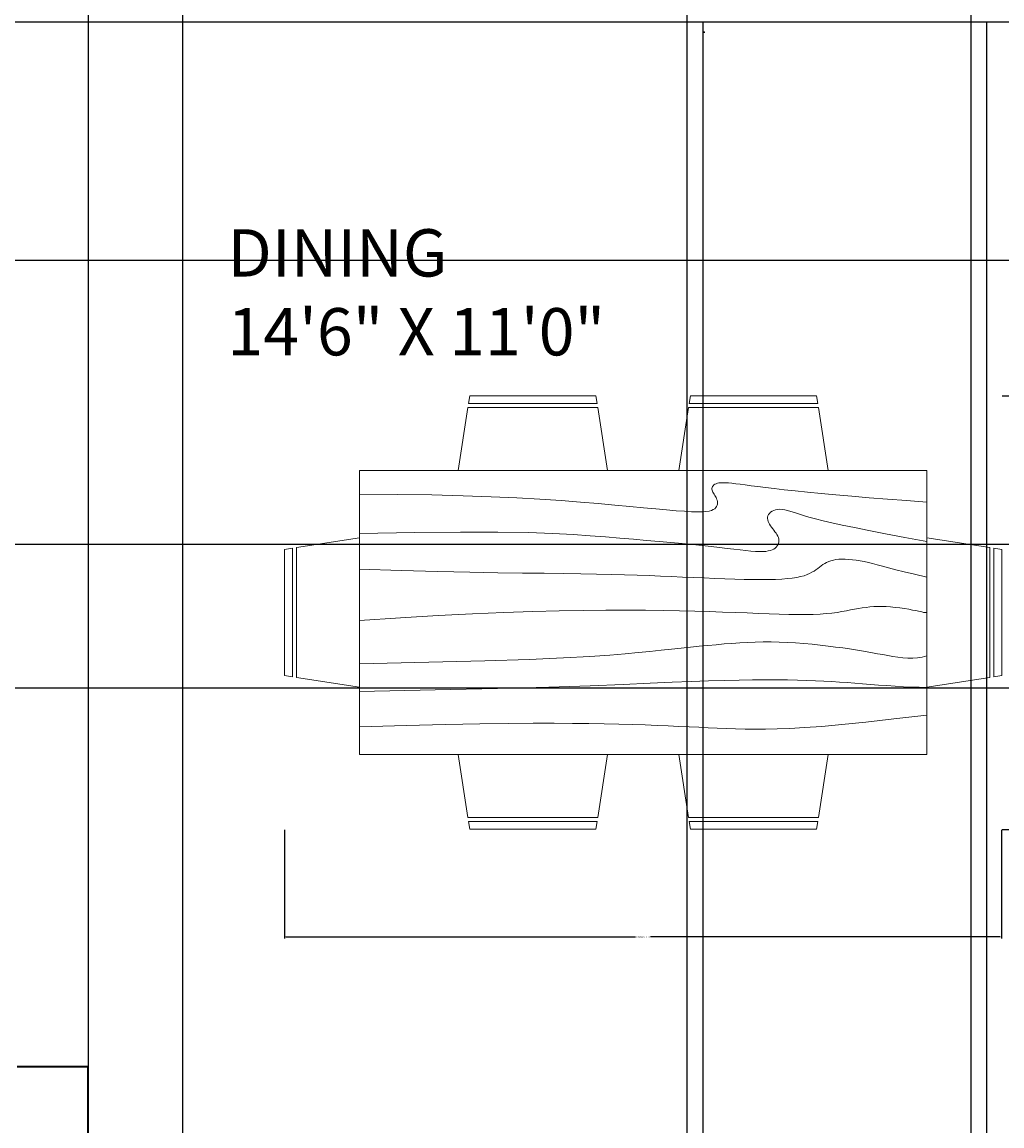
# Model space of a CAD drawing. Units: inches. Extents: x 6662 to 7211, y 5077 to 5683.
# Tile 5 of 9: x 6870 to 6995, y 5325 to 5465. Entities that reach past the tile are written whole.
import ezdxf

# ---------------------------------------------------------------- set-up
doc = ezdxf.new("R2010")
doc.units = ezdxf.units.IN
doc.header["$LTSCALE"] = 3
doc.header["$MEASUREMENT"] = 0
for name, color, linetype, lineweight in [('A-ANNO-DIMS', 2, 'Continuous', 18), ('A-AREA-IDEN', 7, 'Continuous', 18), ('A-FLOR-CASE-PATT', 241, 'Continuous', 13), ('A-FURN', 8, 'Continuous', 18), ('A-WALL', 7, 'Continuous', 35)]:
    doc.layers.add(name, color=color, linetype=linetype, lineweight=lineweight)
doc.styles.get("Standard").update_dxf_attribs({"font": 'arial.ttf'})
doc.dimstyles.get("Standard").update_dxf_attribs({"dimtxt": 0.18, "dimasz": 0.18, "dimexe": 0.18, "dimexo": 0.0625, "dimgap": 0.09, "dimtad": 0, "dimtih": 1, "dimtoh": 1, "dimdec": 4, "dimzin": 0, "dimdsep": 46, "dimtxsty": 'Standard', "dimcen": 0.09, "dimadec": 0, "dimazin": 0, "dimtfac": 1, "dimtdec": 4, "dimtofl": 0, "dimtmove": 0, "dimatfit": 3, "dimfxl": 1, "dimtolj": 1, "dimtzin": 0, "dimarcsym": 0})

# ---------------------------------------------------------------- blocks, each defined once
blk = doc.blocks.new('Dining Set - 36 x 72 in.')
for p, q in [((-22, 27.5), (-22.1562, 26.50042)), ((-22, 27.5), (-6, 27.5)), ((-5.8437, 26.49966), (-6, 27.5)), ((6, 27.5), (5.8438, 26.50042)), ((6, 27.5), (22, 27.5)), ((22.1563, 26.49966), (22, 27.5)), ((-22.2343, 26.00059), (-23.4847, 17.99762)), ((-22.2304, 26), (-5.7608, 26)), ((-5.8416, 26.5), (-22.1534, 26.5)), ((-4.5152, 17.99762), (-5.7655, 25.99926)), ((5.7657, 26.00059), (4.5153, 17.99762)), ((5.7696, 26), (22.2392, 26)), ((22.1584, 26.5), (5.8466, 26.5)), ((23.4848, 17.99762), (22.2345, 25.99926)), ((36, 18), (-36, 18)), ((-36, 18), (-36, -18)), ((36, -18), (36, 18)), ((-44.0006, 8.23428), (-35.9976, 9.48474)), ((44.0006, 8.23428), (35.9976, 9.48474)), ((-45.5, 8), (-44.5004, 8.15617)), ((-45.5, 8), (-45.5, -8)), ((-44.5, -8.15843), (-44.5, 8.15338)), ((-44, 8.23041), (-44, -8.23915)), ((44, 8.23041), (44, -8.23915)), ((44.5, -8.15843), (44.5, 8.15338)), ((45.5, 8), (44.5005, 8.15617)), ((45.5, 8), (45.5, -8)), ((-44.4997, -8.15631), (-45.5, -8)), ((-35.9976, -9.48476), (-43.9993, -8.2345)), ((35.9976, -9.48476), (43.9993, -8.2345)), ((44.4997, -8.15631), (45.5, -8)), ((-36, -18), (36, -18)), ((-22.2343, -26.0006), (-23.4847, -17.99762)), ((-4.5152, -17.99762), (-5.7655, -25.99928)), ((5.7657, -26.0006), (4.5153, -17.99762)), ((23.4848, -17.99762), (22.2345, -25.99928)), ((-22.2304, -26), (-5.7608, -26)), ((-22, -27.5), (-22.1562, -26.50044)), ((-5.8416, -26.5), (-22.1534, -26.5)), ((-5.8437, -26.49967), (-6, -27.5)), ((5.7696, -26), (22.2392, -26)), ((6, -27.5), (5.8438, -26.50044)), ((22.1584, -26.5), (5.8466, -26.5)), ((22.1563, -26.49967), (22, -27.5)), ((-22, -27.5), (-6, -27.5)), ((6, -27.5), (22, -27.5))]:
    blk.add_line(p, q)
for points in [[(-36, 15), (-31.1772, 14.97754), (-26.8079, 14.91406), (-22.8538, 14.81543), (-19.276, 14.6875), (-16.0362, 14.53613), (-13.0957, 14.36718), (-10.4159, 14.18652), (-7.9583, 14), (-5.6904, 13.81315), (-3.6035, 13.63021), (-1.6954, 13.45508), (0.0365, 13.29166), (1.5945, 13.14388), (2.9811, 13.01562), (4.1988, 12.9108), (5.25, 12.83333), (6.1393, 12.78613), (6.8802, 12.76823), (7.4883, 12.77767), (7.9792, 12.8125), (8.3685, 12.87077), (8.6719, 12.95052), (8.9049, 13.0498), (9.0833, 13.16666), (9.2205, 13.29899), (9.3216, 13.44401), (9.3895, 13.59879), (9.4271, 13.76041), (9.4373, 13.92594), (9.4232, 14.09245), (9.3875, 14.257), (9.3333, 14.41666), (9.2638, 14.56917), (9.1836, 14.71484), (9.0975, 14.85465), (9.0104, 14.98958), (8.9272, 15.1206), (8.8529, 15.2487), (8.7922, 15.37483), (8.75, 15.5), (8.7305, 15.62467), (8.7344, 15.74739), (8.7617, 15.86621), (8.8125, 15.97916), (8.8867, 16.08431), (8.9844, 16.17968), (9.1055, 16.26334), (9.25, 16.33333), (9.4189, 16.38802), (9.6172, 16.42708), (9.8506, 16.45052), (10.125, 16.45833), (10.4463, 16.45052), (10.8203, 16.42708), (11.2529, 16.38802), (11.75, 16.33333), (12.3184, 16.26318), (12.9694, 16.17838), (13.7151, 16.07991), (14.5677, 15.96875), (15.5395, 15.84586), (16.6426, 15.71224), (17.8893, 15.56884), (19.2917, 15.41666), (20.859, 15.25667), (22.5879, 15.08984), (24.4721, 14.91715), (26.5052, 14.73958), (28.6809, 14.5581), (30.9929, 14.3737), (33.4347, 14.18733), (36, 14)], [(-36, 10), (-28.9766, 10.14274), (-23.1725, 10.20442), (-18.4241, 10.19775), (-14.5677, 10.13541), (-11.4399, 10.03011), (-8.877, 9.89453), (-6.7154, 9.74137), (-4.7917, 9.58333), (-2.9698, 9.43082), (-1.2246, 9.28515), (0.4415, 9.14534), (2.026, 9.01041), (3.5266, 8.87939), (4.9408, 8.7513), (6.266, 8.62516), (7.5, 8.5), (8.6411, 8.37549), (9.6914, 8.2539), (10.6538, 8.13818), (11.5312, 8.03125), (12.3267, 7.93603), (13.043, 7.85547), (13.6831, 7.79248), (14.25, 7.75), (14.7471, 7.7303), (15.1797, 7.73307), (15.5537, 7.75732), (15.875, 7.80208), (16.1494, 7.86637), (16.3828, 7.94922), (16.5811, 8.04964), (16.75, 8.16666), (16.8944, 8.29915), (17.0143, 8.44531), (17.1089, 8.60319), (17.1771, 8.77083), (17.218, 8.94629), (17.2305, 9.1276), (17.2137, 9.31282), (17.1667, 9.5), (17.0895, 9.6875), (16.987, 9.875), (16.8649, 10.0625), (16.7292, 10.25), (16.5856, 10.4375), (16.4401, 10.625), (16.2985, 10.8125), (16.1667, 11), (16.05, 11.18733), (15.9518, 11.3737), (15.8752, 11.5581), (15.8229, 11.73958), (15.798, 11.91715), (15.8034, 12.08984), (15.842, 12.25667), (15.9167, 12.41666), (16.0295, 12.56836), (16.1784, 12.70833), (16.3605, 12.83268), (16.5729, 12.9375), (16.8127, 13.01888), (17.0768, 13.07291), (17.3625, 13.0957), (17.6667, 13.08333), (17.9894, 13.03312), (18.3418, 12.94726), (18.7382, 12.82918), (19.1927, 12.68229), (19.7195, 12.51001), (20.3327, 12.31575), (21.0465, 12.10294), (21.875, 11.875), (22.8357, 11.63354), (23.959, 11.37304), (25.2786, 11.08618), (26.8282, 10.76562), (28.6414, 10.40405), (30.752, 9.99414), (33.1936, 9.52856), (36, 9)], [(-36, 5.5), (-30.7157, 5.3348), (-26.069, 5.20963), (-21.9946, 5.11767), (-18.4271, 5.05208), (-15.3009, 5.00602), (-12.5508, 4.97265), (-10.1112, 4.94515), (-7.9167, 4.91666), (-5.909, 4.88167), (-4.0586, 4.83984), (-2.3429, 4.79215), (-0.7396, 4.73958), (0.7739, 4.6831), (2.22, 4.6237), (3.6213, 4.56233), (5, 4.5), (6.373, 4.43782), (7.7344, 4.3776), (9.0723, 4.32129), (10.375, 4.27083), (11.6309, 4.22819), (12.8281, 4.19531), (13.9551, 4.17415), (15, 4.16666), (15.954, 4.17448), (16.819, 4.19791), (17.6001, 4.23698), (18.3021, 4.29166), (18.9299, 4.36198), (19.4883, 4.44791), (19.9823, 4.54948), (20.4167, 4.66666), (20.7969, 4.79899), (21.1302, 4.94401), (21.4245, 5.09879), (21.6875, 5.26041), (21.9271, 5.42594), (22.1511, 5.59245), (22.3672, 5.757), (22.5834, 5.91666), (22.8065, 6.06868), (23.0404, 6.21093), (23.2879, 6.34147), (23.5521, 6.45833), (23.8358, 6.55957), (24.142, 6.64323), (24.4735, 6.70735), (24.8334, 6.75), (25.2235, 6.76969), (25.642, 6.76692), (26.0858, 6.74267), (26.5521, 6.69791), (27.0379, 6.63362), (27.5404, 6.55078), (28.0565, 6.45036), (28.5834, 6.33333), (29.1242, 6.19987), (29.7071, 6.04687), (30.3661, 5.87044), (31.1354, 5.66666), (32.0493, 5.43164), (33.142, 5.16146), (34.4475, 4.85221), (36, 4.5)], [(-36, -1), (-30.7915, -0.6591), (-26.0195, -0.38216), (-21.6519, -0.16284), (-17.6563, 0.00521), (-14.0005, 0.12833), (-10.6523, 0.21289), (-7.5796, 0.26522), (-4.75, 0.29166), (-2.134, 0.29793), (0.2878, 0.28711), (2.5317, 0.26163), (4.6146, 0.22396), (6.5529, 0.17651), (8.3633, 0.12174), (10.0623, 0.06209), (11.6667, 0), (13.1899, -0.06201), (14.6341, -0.1211), (15.9982, -0.17432), (17.2813, -0.21875), (18.4823, -0.25147), (19.6003, -0.26953), (20.6343, -0.27002), (21.5834, -0.25), (22.4481, -0.20768), (23.2357, -0.14584), (23.9549, -0.06836), (24.6146, 0.02083), (25.2235, 0.11784), (25.7904, 0.21875), (26.3241, 0.31966), (26.8334, 0.41666), (27.3265, 0.50618), (27.8099, 0.58593), (28.2894, 0.65397), (28.7709, 0.70833), (29.2601, 0.74707), (29.763, 0.76823), (30.2855, 0.76985), (30.8334, 0.75), (31.4088, 0.70784), (31.9994, 0.64713), (32.589, 0.57275), (33.1615, 0.48958), (33.7008, 0.4025), (34.1908, 0.3164), (34.6153, 0.23616), (34.9584, 0.16666), (35.2099, 0.11165), (35.3848, 0.07031), (35.504, 0.04069), (35.5886, 0.02083), (35.6594, 0.00879), (35.7377, 0.0026), (35.8442, 0.00032), (36, 0)], [(-36, -6.5), (-27.1843, -6.31267), (-20.084, -6.1263), (-14.469, -5.9419), (-10.1094, -5.76042), (-6.7752, -5.58285), (-4.2363, -5.41016), (-2.2629, -5.24333), (-0.625, -5.08334), (0.8708, -4.93099), (2.2715, -4.78646), (3.5872, -4.64974), (4.8281, -4.52084), (6.0046, -4.39974), (7.127, -4.28646), (8.2053, -4.18099), (9.25, -4.08334), (10.2705, -3.99382), (11.2734, -3.91407), (12.2647, -3.84603), (13.25, -3.79167), (14.2354, -3.75293), (15.2266, -3.73177), (16.2295, -3.73015), (17.25, -3.75), (18.2912, -3.79248), (19.3451, -3.85547), (20.4009, -3.93604), (21.4479, -4.03125), (22.4754, -4.13819), (23.4727, -4.25391), (24.4289, -4.37549), (25.3334, -4.5), (26.1785, -4.62492), (26.9694, -4.74935), (27.7145, -4.87281), (28.4219, -4.99479), (29.1, -5.11483), (29.7572, -5.23242), (30.4016, -5.34709), (31.0417, -5.45834), (31.6837, -5.56437), (32.3262, -5.65821), (32.9658, -5.73153), (33.599, -5.77604), (34.2224, -5.78345), (34.8327, -5.74545), (35.4264, -5.65373), (36, -5.5)], [(-36, -10), (-26.4022, -9.81299), (-18.4675, -9.62891), (-11.9839, -9.45069), (-6.7396, -9.28125), (-2.5226, -9.12354), (0.8789, -8.98047), (3.6769, -8.85498), (6.0833, -8.75), (8.2767, -8.66765), (10.3021, -8.60677), (12.1712, -8.56543), (13.8958, -8.54167), (15.4876, -8.53353), (16.9583, -8.53907), (18.3197, -8.55632), (19.5834, -8.58334), (20.7616, -8.61841), (21.8685, -8.66081), (22.9188, -8.71004), (23.9271, -8.76563), (24.9081, -8.82707), (25.8763, -8.89388), (26.8465, -8.96558), (27.8334, -9.04167), (28.8474, -9.12118), (29.8828, -9.20117), (30.93, -9.27824), (31.9792, -9.34896), (33.0205, -9.40991), (34.0443, -9.45768), (35.0407, -9.48885), (36, -9.5)], [(-36, -14.5), (-30.0881, -14.33513), (-25.0332, -14.21224), (-20.7312, -14.12647), (-17.0781, -14.07292), (-13.97, -14.04671), (-11.3027, -14.04297), (-8.9724, -14.05681), (-6.875, -14.08334), (-4.9224, -14.11833), (-3.0905, -14.16016), (-1.3709, -14.20785), (0.2448, -14.26042), (1.7647, -14.3169), (3.1973, -14.3763), (4.5507, -14.43767), (5.8333, -14.5), (7.0554, -14.5621), (8.235, -14.62175), (9.3922, -14.67652), (10.5469, -14.72396), (11.7192, -14.76164), (12.929, -14.78711), (14.1965, -14.79794), (15.5417, -14.79167), (16.9933, -14.76424), (18.6152, -14.70508), (20.4804, -14.60197), (22.6615, -14.44271), (25.2312, -14.21509), (28.2624, -13.9069), (31.8277, -13.50594), (36, -13)]]:
    blk.add_lwpolyline(points)
blk = doc.blocks.new('*D38')
at = {"layer": 'A-ANNO-DIMS', "color": 0, "lineweight": -2, "ltscale": 3, "transparency": 16777216}
for p, q in [((6903.79, 5362.15), (6903.79, 5348.38)), ((6994.79, 5362.15), (6994.79, 5348.38)), ((6903.97, 5348.56), (6948.34, 5348.56)), ((6994.61, 5348.56), (6950.24, 5348.56))]:
    blk.add_line(p, q, dxfattribs=at)
at = {"layer": 'A-ANNO-DIMS', "color": 0, "ltscale": 3, "transparency": 16777216}
for points in [[(6903.97, 5348.59), (6903.97, 5348.53), (6903.79, 5348.56)], [(6994.61, 5348.59), (6994.61, 5348.53), (6994.79, 5348.56)]]:
    blk.add_solid(points, dxfattribs=at)
at = {"layer": 'Defpoints', "color": 0, "ltscale": 3, "transparency": 16777216}
for p in [(6903.79, 5362.21), (6994.79, 5362.21), (6994.79, 5348.56)]:
    blk.add_point(p, dxfattribs=at)
at = {"layer": 'A-ANNO-DIMS', "color": 0, "ltscale": 3, "transparency": 16777216, "insert": (6949.29, 5348.56), "char_height": 0.18, "attachment_point": 5}
blk.add_mtext('\\A1;DINING SET 91', dxfattribs=at)
blk = doc.blocks.new('*D39')
at = {"layer": 'A-ANNO-DIMS', "color": 0, "lineweight": -2, "ltscale": 3, "transparency": 16777216}
for p, q in [((6994.86, 5417.21), (7008.62, 5417.21)), ((7008.44, 5417.03), (7008.44, 5389.9)), ((7008.44, 5362.39), (7008.44, 5389.53)), ((6994.86, 5362.21), (7008.62, 5362.21))]:
    blk.add_line(p, q, dxfattribs=at)
at = {"layer": 'A-ANNO-DIMS', "color": 0, "ltscale": 3, "transparency": 16777216}
for points in [[(7008.41, 5417.03), (7008.47, 5417.03), (7008.44, 5417.21)], [(7008.41, 5362.39), (7008.47, 5362.39), (7008.44, 5362.21)]]:
    blk.add_solid(points, dxfattribs=at)
at = {"layer": 'Defpoints', "color": 0, "ltscale": 3, "transparency": 16777216}
for p in [(6994.79, 5417.21), (7008.44, 5417.21), (6994.79, 5362.21)]:
    blk.add_point(p, dxfattribs=at)
at = {"layer": 'A-ANNO-DIMS', "color": 0, "ltscale": 3, "transparency": 16777216, "insert": (7008.44, 5389.71), "char_height": 0.18, "attachment_point": 5}
blk.add_mtext('\\A1;55', dxfattribs=at)
blk = doc.blocks.new('*D40')
at = {"layer": 'A-ANNO-DIMS', "color": 0, "lineweight": -2, "ltscale": 3, "transparency": 16777216}
for p, q in [((7182.86, 5326.04), (7182.86, 5076.72)), ((6689.86, 5323.04), (6689.86, 5076.72)), ((6690.04, 5076.9), (6936.07, 5076.9)), ((7182.68, 5076.9), (6936.65, 5076.9))]:
    blk.add_line(p, q, dxfattribs=at)
at = {"layer": 'A-ANNO-DIMS', "color": 0, "ltscale": 3, "transparency": 16777216}
for points in [[(6690.04, 5076.93), (6690.04, 5076.87), (6689.86, 5076.9)], [(7182.68, 5076.93), (7182.68, 5076.87), (7182.86, 5076.9)]]:
    blk.add_solid(points, dxfattribs=at)
at = {"layer": 'Defpoints', "color": 0, "ltscale": 3, "transparency": 16777216}
for p in [(7182.86, 5326.1), (6689.86, 5323.1), (7182.86, 5076.9)]:
    blk.add_point(p, dxfattribs=at)
at = {"layer": 'A-ANNO-DIMS', "color": 0, "ltscale": 3, "transparency": 16777216, "insert": (6936.36, 5076.9), "char_height": 0.18, "attachment_point": 5}
blk.add_mtext('\\A1;493', dxfattribs=at)
blk = doc.blocks.new('*D61')
at = {"layer": 'A-ANNO-DIMS', "color": 0, "lineweight": -2, "ltscale": 3, "transparency": 16777216}
for p, q in [((7167.8, 5434.35), (6661.98, 5434.35)), ((6662.16, 5434.17), (6662.16, 5416.53)), ((6662.16, 5398.53), (6662.16, 5416.17)), ((7167.8, 5398.35), (6661.98, 5398.35))]:
    blk.add_line(p, q, dxfattribs=at)
at = {"layer": 'A-ANNO-DIMS', "color": 0, "ltscale": 3, "transparency": 16777216}
for points in [[(6662.13, 5434.17), (6662.19, 5434.17), (6662.16, 5434.35)], [(6662.13, 5398.53), (6662.19, 5398.53), (6662.16, 5398.35)]]:
    blk.add_solid(points, dxfattribs=at)
at = {"layer": 'Defpoints', "color": 0, "ltscale": 3, "transparency": 16777216}
for p in [(6662.16, 5434.35), (7167.86, 5434.35), (7167.86, 5398.35)]:
    blk.add_point(p, dxfattribs=at)
at = {"layer": 'A-ANNO-DIMS', "color": 0, "ltscale": 3, "transparency": 16777216, "insert": (6662.16, 5416.35), "char_height": 0.18, "attachment_point": 5}
blk.add_mtext('\\A1;36', dxfattribs=at)
blk = doc.blocks.new('*D66')
at = {"layer": 'A-ANNO-DIMS', "color": 0, "lineweight": -2, "ltscale": 3, "transparency": 16777216}
for p, q in [((6956.86, 5464.54), (6956.86, 5076.72)), ((6992.86, 5464.54), (6992.86, 5076.72)), ((6957.04, 5076.9), (6974.64, 5076.9)), ((6992.68, 5076.9), (6975.08, 5076.9))]:
    blk.add_line(p, q, dxfattribs=at)
at = {"layer": 'A-ANNO-DIMS', "color": 0, "ltscale": 3, "transparency": 16777216}
for points in [[(6957.04, 5076.93), (6957.04, 5076.87), (6956.86, 5076.9)], [(6992.68, 5076.93), (6992.68, 5076.87), (6992.86, 5076.9)]]:
    blk.add_solid(points, dxfattribs=at)
at = {"layer": 'Defpoints', "color": 0, "ltscale": 3, "transparency": 16777216}
for p in [(6956.86, 5464.6), (6992.86, 5464.6), (6992.86, 5076.9)]:
    blk.add_point(p, dxfattribs=at)
at = {"layer": 'A-ANNO-DIMS', "color": 0, "ltscale": 3, "transparency": 16777216, "insert": (6974.86, 5076.9), "char_height": 0.18, "attachment_point": 5}
blk.add_mtext('\\A1;36', dxfattribs=at)
blk = doc.blocks.new('*D71')
at = {"layer": 'A-ANNO-DIMS', "color": 0, "lineweight": -2, "ltscale": 3, "transparency": 16777216}
for p, q in [((6878.86, 5617.54), (6878.86, 5076.72)), ((6890.86, 5617.54), (6890.86, 5076.72)), ((6879.04, 5076.9), (6884.65, 5076.9)), ((6890.68, 5076.9), (6885.07, 5076.9))]:
    blk.add_line(p, q, dxfattribs=at)
at = {"layer": 'A-ANNO-DIMS', "color": 0, "ltscale": 3, "transparency": 16777216}
for points in [[(6879.04, 5076.93), (6879.04, 5076.87), (6878.86, 5076.9)], [(6890.68, 5076.93), (6890.68, 5076.87), (6890.86, 5076.9)]]:
    blk.add_solid(points, dxfattribs=at)
at = {"layer": 'Defpoints', "color": 0, "ltscale": 3, "transparency": 16777216}
for p in [(6878.86, 5617.6), (6890.86, 5617.6), (6878.86, 5076.9)]:
    blk.add_point(p, dxfattribs=at)
at = {"layer": 'A-ANNO-DIMS', "color": 0, "ltscale": 3, "transparency": 16777216, "insert": (6884.86, 5076.9), "char_height": 0.18, "attachment_point": 5}
blk.add_mtext('\\A1;12', dxfattribs=at)
blk = doc.blocks.new('*D72')
at = {"layer": 'A-ANNO-DIMS', "color": 0, "lineweight": -2, "ltscale": 3, "transparency": 16777216}
for p, q in [((6954.86, 5617.54), (6954.86, 5076.72)), ((6990.86, 5617.54), (6990.86, 5076.72)), ((6955.04, 5076.9), (6972.64, 5076.9)), ((6990.68, 5076.9), (6973.08, 5076.9))]:
    blk.add_line(p, q, dxfattribs=at)
at = {"layer": 'A-ANNO-DIMS', "color": 0, "ltscale": 3, "transparency": 16777216}
for points in [[(6955.04, 5076.93), (6955.04, 5076.87), (6954.86, 5076.9)], [(6990.68, 5076.93), (6990.68, 5076.87), (6990.86, 5076.9)]]:
    blk.add_solid(points, dxfattribs=at)
at = {"layer": 'Defpoints', "color": 0, "ltscale": 3, "transparency": 16777216}
for p in [(6954.86, 5617.6), (6990.86, 5617.6), (6990.86, 5076.9)]:
    blk.add_point(p, dxfattribs=at)
at = {"layer": 'A-ANNO-DIMS', "color": 0, "ltscale": 3, "transparency": 16777216, "insert": (6972.86, 5076.9), "char_height": 0.18, "attachment_point": 5}
blk.add_mtext('\\A1;36', dxfattribs=at)
blk = doc.blocks.new('*D76')
at = {"layer": 'A-ANNO-DIMS', "color": 0, "lineweight": -2, "ltscale": 3, "transparency": 16777216}
for p, q in [((7167.8, 5464.6), (6661.98, 5464.6)), ((6662.16, 5464.42), (6662.16, 5449.65)), ((6662.16, 5434.53), (6662.16, 5449.29)), ((7167.8, 5434.35), (6661.98, 5434.35))]:
    blk.add_line(p, q, dxfattribs=at)
at = {"layer": 'A-ANNO-DIMS', "color": 0, "ltscale": 3, "transparency": 16777216}
for points in [[(6662.13, 5464.42), (6662.19, 5464.42), (6662.16, 5464.6)], [(6662.13, 5434.53), (6662.19, 5434.53), (6662.16, 5434.35)]]:
    blk.add_solid(points, dxfattribs=at)
at = {"layer": 'Defpoints', "color": 0, "ltscale": 3, "transparency": 16777216}
for p in [(7167.86, 5464.6), (6662.16, 5434.35), (7167.86, 5434.35)]:
    blk.add_point(p, dxfattribs=at)
at = {"layer": 'A-ANNO-DIMS', "color": 0, "ltscale": 3, "transparency": 16777216, "insert": (6662.16, 5449.47), "char_height": 0.18, "attachment_point": 5}
blk.add_mtext('\\A1;30.25', dxfattribs=at)
blk = doc.blocks.new('*D77')
at = {"layer": 'A-ANNO-DIMS', "color": 0, "lineweight": -2, "ltscale": 3, "transparency": 16777216}
for p, q in [((7167.8, 5398.35), (6661.98, 5398.35)), ((6662.16, 5398.17), (6662.16, 5389.4)), ((6662.16, 5380.28), (6662.16, 5389.04)), ((7167.8, 5380.1), (6661.98, 5380.1))]:
    blk.add_line(p, q, dxfattribs=at)
at = {"layer": 'A-ANNO-DIMS', "color": 0, "ltscale": 3, "transparency": 16777216}
for points in [[(6662.13, 5398.17), (6662.19, 5398.17), (6662.16, 5398.35)], [(6662.13, 5380.28), (6662.19, 5380.28), (6662.16, 5380.1)]]:
    blk.add_solid(points, dxfattribs=at)
at = {"layer": 'Defpoints', "color": 0, "ltscale": 3, "transparency": 16777216}
for p in [(7167.86, 5398.35), (6662.16, 5380.1), (7167.86, 5380.1)]:
    blk.add_point(p, dxfattribs=at)
at = {"layer": 'A-ANNO-DIMS', "color": 0, "ltscale": 3, "transparency": 16777216, "insert": (6662.16, 5389.22), "char_height": 0.18, "attachment_point": 5}
blk.add_mtext('\\A1;18.25', dxfattribs=at)
blk = doc.blocks.new('*D88')
at = {"layer": 'A-ANNO-DIMS', "color": 0, "lineweight": -2, "ltscale": 3, "transparency": 16777216}
for p, q in [((6992.81, 5511.04), (6979.5, 5493.29)), ((6992.99, 5511.04), (6992.81, 5511.04)), ((6956.93, 5463.31), (6957.11, 5463.31)), ((6957.02, 5463.22), (6957.02, 5463.4))]:
    blk.add_line(p, q, dxfattribs=at)
at = {"layer": 'A-ANNO-DIMS', "color": 0, "ltscale": 3, "transparency": 16777216}
blk.add_solid([(6979.47, 5493.3), (6979.52, 5493.27), (6979.39, 5493.14)], dxfattribs=at)
at = {"layer": 'Defpoints', "color": 0, "ltscale": 3, "transparency": 16777216}
for p in [(6979.39, 5493.14), (6957.02, 5463.31)]:
    blk.add_point(p, dxfattribs=at)
at = {"layer": 'A-ANNO-DIMS', "color": 0, "ltscale": 3, "transparency": 16777216, "insert": (6993.54, 5511.04), "char_height": 0.18, "attachment_point": 5}
blk.add_mtext('\\A1;R37.285', dxfattribs=at)

msp = doc.modelspace()

# ---------------------------------------------------------------- hatches: boundary and pattern name
at = {"layer": 'A-FLOR-CASE-PATT'}
h = msp.add_hatch(dxfattribs=at)
h.set_pattern_fill('ANSI31', color=256)
h.paths.add_polyline_path([(6869.8579, 5283.7981), (6845.8579, 5283.7981), (6845.8579, 5229.4653), (6847.018, 5229.7817, -0.54116316), (6849.0925, 5228.1371), (6849.7129, 5228.234, -0.50821327), (6851.018, 5227.2817), (6851.018, 5226.7817), (6855.018, 5227.2817), (6855.018, 5225.7817), (6851.018, 5225.2817), (6851.018, 5217.7817), (6851.018, 5210.2817), (6855.018, 5209.7817), (6855.018, 5208.2817), (6851.018, 5208.7817), (6851.018, 5208.2817, -0.41421356), (6850.018, 5207.2817), (6849.0925, 5207.4263, -0.50580924), (6847.1872, 5205.7355), (6845.8579, 5206.0981), (6845.8579, 5179.0979), (6869.8579, 5179.0979)])
h.paths.add_polyline_path([(7167.8579, 5497.5979), (7143.8579, 5497.5979), (7078.3579, 5497.5979), (7078.3579, 5473.5979), (7163.8579, 5473.5979), (7167.8579, 5473.5979)])
h.paths.add_polyline_path([(6825.9016, 5497.5979), (6725.8579, 5497.5979), (6725.8579, 5473.5979), (6825.9016, 5473.5979)])
h.paths.add_polyline_path([(6796.6359, 5485.2095), (6797.1359, 5489.2095), (6806.1359, 5489.2095), (6815.1359, 5489.2095), (6815.6359, 5485.2095), (6814.1359, 5485.2095), (6813.6359, 5489.2095), (6806.1359, 5489.2095), (6798.6359, 5489.2095), (6798.1359, 5485.2095)], flags=16)

# ---------------------------------------------------------------- linework, layer by layer
at = {"layer": 'A-WALL'}
for p, q in [((6878.8579, 5332.0979), (6869.8579, 5332.0979)), ((6878.8579, 5202.5979), (6878.8579, 5332.0979))]:
    msp.add_line(p, q, dxfattribs=at)

# ---------------------------------------------------------------- block references
at = {"layer": 'A-FURN'}
msp.add_blockref('Dining Set - 36 x 72 in.', (6949.2933, 5389.7146), dxfattribs=at)

# ---------------------------------------------------------------- texts
at = {"layer": 'A-AREA-IDEN', "ltscale": 3, "insert": (6896.5433, 5438.3242), "char_height": 6, "attachment_point": 1}
msp.add_mtext_dynamic_manual_height_columns('DINING\\P14\'6" X 11\'0"', width=381.547883, gutter_width=1, heights=[0], dxfattribs=at)

# ---------------------------------------------------------------- dimensions: what is measured, and where the dimension line sits
at = {"layer": 'A-ANNO-DIMS', "ltscale": 3}
for base, p1, p2, picture, middle in [((6878.8579, 5076.8979), (6890.8579, 5617.5979), (6878.8579, 5617.5979), '*D71', (6884.8579, 5076.8979)), ((6990.8579, 5076.8979), (6954.8579, 5617.5979), (6990.8579, 5617.5979), '*D72', (6972.8579, 5076.8979)), ((6992.8579, 5076.8979), (6956.8579, 5464.5979), (6992.8579, 5464.5979), '*D66', (6974.8579, 5076.8979)), ((7182.8579, 5076.8979), (6689.8579, 5323.0979), (7182.8579, 5326.0979), '*D40', (6936.3579, 5076.8979))]:
    dim = msp.add_linear_dim(base=base, p1=p1, p2=p2, dimstyle='Standard', override={"dimdec": 0, "dimlfac": 1, "dimrnd": 0, "dimzin": 0, "dimdsep": 46, "dimlunit": 2}, dxfattribs=at)
    dim.commit()
    dim.dimension.update_dxf_attribs({"geometry": picture, "text_midpoint": middle})
dim = msp.add_radius_dim(center=(6957.0195, 5463.3135), mpoint=(6979.3903, 5493.1414), dimstyle='Standard', override={"dimdec": 3, "dimlfac": 1, "dimrnd": 0, "dimzin": 0, "dimdsep": 46, "dimlunit": 2}, dxfattribs=at)
dim.commit()
dim.dimension.update_dxf_attribs({"geometry": '*D88', "text_midpoint": (6993.5432, 5511.0382), "dimtype": 164})
for base, p1, p2, override, picture, middle in [((6662.1579, 5434.3479), (7167.8579, 5464.5979), (7167.8579, 5434.3479), {"dimdec": 2, "dimlfac": 1, "dimrnd": 0, "dimzin": 0, "dimdsep": 46, "dimlunit": 2}, '*D76', (6662.1579, 5449.4729)), ((6662.1579, 5434.3479), (7167.8579, 5398.3479), (7167.8579, 5434.3479), {"dimdec": 0, "dimlfac": 1, "dimrnd": 0, "dimzin": 0, "dimdsep": 46, "dimlunit": 2}, '*D61', (6662.1579, 5416.3479)), ((7008.4433, 5417.2146), (6994.7933, 5362.2146), (6994.7933, 5417.2146), {"dimdec": 0, "dimlfac": 1, "dimrnd": 0, "dimzin": 0, "dimdsep": 46, "dimlunit": 2}, '*D39', (7008.4433, 5389.7146)), ((6662.1579, 5380.0979), (7167.8579, 5398.3479), (7167.8579, 5380.0979), {"dimdec": 2, "dimlfac": 1, "dimrnd": 0, "dimzin": 0, "dimdsep": 46, "dimlunit": 2}, '*D77', (6662.1579, 5389.2229))]:
    dim = msp.add_linear_dim(base=base, p1=p1, p2=p2, angle=90, dimstyle='Standard', override=override, dxfattribs=at)
    dim.commit()
    dim.dimension.update_dxf_attribs({"geometry": picture, "text_midpoint": middle})
dim = msp.add_linear_dim(base=(6994.7933, 5348.5646), p1=(6903.7933, 5362.2146), p2=(6994.7933, 5362.2146), text='DINING SET <>', dimstyle='Standard', override={"dimdec": 0, "dimlfac": 1, "dimrnd": 0, "dimzin": 0, "dimdsep": 46, "dimlunit": 2}, dxfattribs=at)
dim.commit()
dim.dimension.update_dxf_attribs({"geometry": '*D38', "text_midpoint": (6949.2933, 5348.5646)})

doc.saveas('drawing.dxf')
